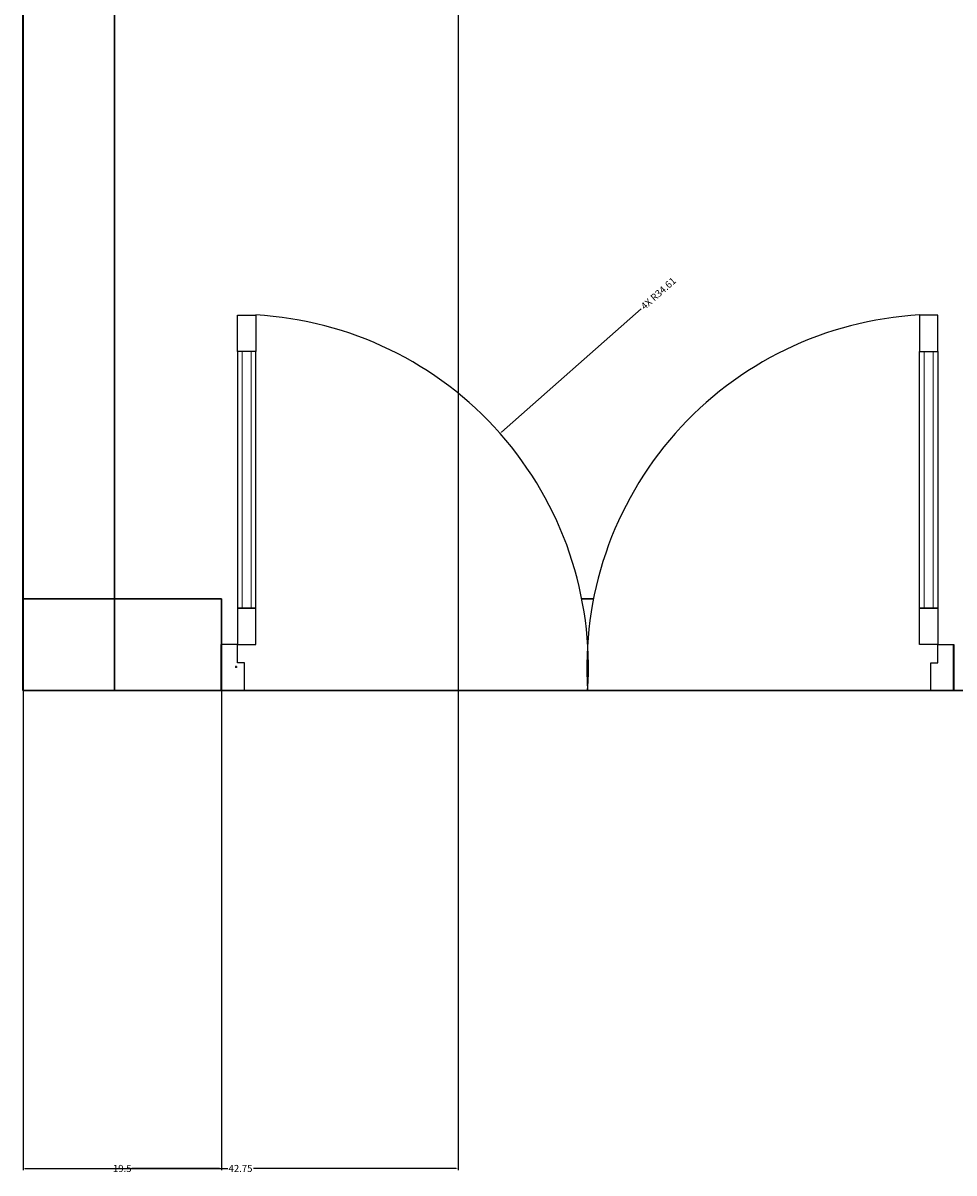
# Model space of a CAD drawing. Units: inches. Extents: x 867 to 1667, y -234 to 788.
# Tile 1 of 42: x 915 to 1006, y -234 to -121. Entities that reach past the tile are written whole.
import ezdxf

# ---------------------------------------------------------------- set-up
doc = ezdxf.new("R2010")
doc.units = ezdxf.units.IN
doc.header["$MEASUREMENT"] = 0
for name, color, linetype, lineweight in [('A-ANNO-DIMS', 2, 'Continuous', 18), ('A-Door', 150, 'Continuous', 25), ('A-Glaz', 92, 'Continuous', 18), ('A-Wall', 7, 'Continuous', 35), ('A-WALL-SITE', 8, 'Continuous', 30)]:
    doc.layers.add(name, color=color, linetype=linetype, lineweight=lineweight)
doc.layers.add('NT', color=1, linetype='Continuous')
doc.styles.get("Standard").update_dxf_attribs({"font": 'arial.ttf'})
doc.dimstyles.get("Standard").update_dxf_attribs({"dimtxt": 0.6875, "dimasz": 0.18, "dimexe": 0.18, "dimexo": 0.0625, "dimgap": 0.09, "dimtad": 0, "dimdec": 4, "dimzin": 0, "dimdsep": 46, "dimlunit": 4, "dimtxsty": 'Standard', "dimcen": 0.09, "dimadec": 0, "dimazin": 0, "dimtfac": 1, "dimtdec": 4, "dimtofl": 0, "dimtmove": 0, "dimatfit": 3, "dimfxl": 1, "dimtolj": 1, "dimtzin": 0, "dimarcsym": 0})

# ---------------------------------------------------------------- blocks, each defined once
blk = doc.blocks.new('A$C0EE93B68')
at = {"layer": 'A-Door'}
for points in [[(100, 1565), (100, 1600), (0, 1600), (0, 1550), (50, 1550), (60, 1550), (60, 1565)], [(100, 1525), (180, 1525), (180, 1565), (100, 1565)], [(180, 1525), (740, 1525), (740, 1565), (180, 1565)], [(820, 1525), (740, 1525), (740, 1565), (820, 1565)], [(100, 75), (180, 75), (180, 35), (100, 35)], [(180, 75), (740, 75), (740, 35), (180, 35)], [(820, 75), (740, 75), (740, 35), (820, 35)], [(100, 35), (100, 0), (0, 0), (0, 50), (50, 50), (60, 50), (60, 35)]]:
    blk.add_lwpolyline(points, close=True, dxfattribs=at)
at = {"layer": 'A-Glaz'}
for points in [[(180, 1535), (740, 1535), (740, 1555), (180, 1555)], [(180, 65), (740, 65), (740, 45), (180, 45)]]:
    blk.add_lwpolyline(points, close=True, dxfattribs=at)
at = {"layer": 'A-Wall'}
for p, q in [((0, 1600), (100, 1600)), ((0, 0), (100, 0))]:
    blk.add_line(p, q, dxfattribs=at)
at = {"layer": 'NT'}
for centre, start, end in [((51.6, 1567.9), 266.1547, 356.8081), ((51.6, 32.1), 3.1919, 93.8453)]:
    blk.add_arc(centre, 769.6, start, end, dxfattribs=at)
blk = doc.blocks.new('*D26')
at = {"layer": 'A-ANNO-DIMS', "color": 0, "lineweight": -2, "transparency": 16777216}
for p, q in [((914.89, -186.47), (914.89, -233.54)), ((934.39, -186.47), (934.39, -233.54)), ((915.07, -233.36), (923.68, -233.36)), ((934.21, -233.36), (925.59, -233.36))]:
    blk.add_line(p, q, dxfattribs=at)
at = {"layer": 'A-ANNO-DIMS', "color": 0, "transparency": 16777216}
for points in [[(915.07, -233.33), (915.07, -233.39), (914.89, -233.36)], [(934.21, -233.33), (934.21, -233.39), (934.39, -233.36)]]:
    blk.add_solid(points, dxfattribs=at)
at = {"layer": 'Defpoints', "color": 0, "transparency": 16777216}
for p in [(914.89, -186.41), (934.39, -186.41), (914.89, -233.36)]:
    blk.add_point(p, dxfattribs=at)
at = {"layer": 'A-ANNO-DIMS', "color": 0, "transparency": 16777216, "insert": (924.64, -233.36), "char_height": 0.688, "attachment_point": 5}
blk.add_mtext('\\A1;19.5', dxfattribs=at)
blk = doc.blocks.new('*D28')
at = {"layer": 'A-ANNO-DIMS', "color": 0, "lineweight": -2, "transparency": 16777216}
for p, q in [((914.89, 623.55), (914.89, -233.54)), ((957.64, 623.55), (957.64, -233.54)), ((915.07, -233.36), (935, -233.36)), ((957.46, -233.36), (937.53, -233.36))]:
    blk.add_line(p, q, dxfattribs=at)
at = {"layer": 'A-ANNO-DIMS', "color": 0, "transparency": 16777216}
for points in [[(915.07, -233.33), (915.07, -233.39), (914.89, -233.36)], [(957.46, -233.33), (957.46, -233.39), (957.64, -233.36)]]:
    blk.add_solid(points, dxfattribs=at)
at = {"layer": 'Defpoints', "color": 0, "transparency": 16777216}
for p in [(914.89, 623.62), (957.64, 623.62), (914.89, -233.36)]:
    blk.add_point(p, dxfattribs=at)
at = {"layer": 'A-ANNO-DIMS', "color": 0, "transparency": 16777216, "insert": (936.26, -233.36), "char_height": 0.688, "attachment_point": 5}
blk.add_mtext('\\A1;42.75', dxfattribs=at)
blk = doc.blocks.new('*D65')
at = {"layer": 'A-ANNO-DIMS', "color": 0, "lineweight": -2, "transparency": 16777216}
for p, q in [((975.63, -148.91), (961.9, -161.04)), ((935.74, -184.09), (935.92, -184.09)), ((935.83, -184.18), (935.83, -184))]:
    blk.add_line(p, q, dxfattribs=at)
at = {"layer": 'A-ANNO-DIMS', "color": 0, "transparency": 16777216}
blk.add_solid([(961.88, -161.02), (961.92, -161.06), (961.76, -161.16)], dxfattribs=at)
at = {"layer": 'Defpoints', "color": 0, "transparency": 16777216}
for p in [(961.76, -161.16), (935.83, -184.09)]:
    blk.add_point(p, dxfattribs=at)
at = {"layer": 'A-ANNO-DIMS', "color": 0, "transparency": 16777216, "insert": (977.32, -147.41), "char_height": 0.6875, "attachment_point": 5, "rotation": 41.4815}
blk.add_mtext('\\A1;4X R34.61', dxfattribs=at)

msp = doc.modelspace()

# ---------------------------------------------------------------- linework, layer by layer
at = {"layer": 'A-WALL-SITE'}
for p, q in [((914.8866, 740.617), (914.8866, -186.4081)), ((923.8866, 740.617), (923.8866, -186.4081)), ((934.3882, -177.4081), (914.8866, -177.4081)), ((934.3882, -177.4081), (934.3882, -186.4081)), ((934.3882, -177.4081), (934.3882, -186.4081)), ((970.9402, -177.4081), (969.7951, -177.4081)), ((1619.8866, -186.4081), (914.8866, -186.4081))]:
    msp.add_line(p, q, dxfattribs=at)

# ---------------------------------------------------------------- block references
at = {"layer": 'A-Door', "xscale": 0.0449743717352066, "yscale": 0.0449743717352066, "zscale": 0.0449743717352066, "rotation": 90}
msp.add_blockref('A$C0EE93B68', (1006.3472, -186.4081), dxfattribs=at)

# ---------------------------------------------------------------- dimensions: what is measured, and where the dimension line sits
at = {"layer": 'A-ANNO-DIMS'}
for p1, p2, override, picture, middle in [((957.6375, 623.617), (914.8866, 623.617), {"dimdec": 2, "dimlfac": 1, "dimrnd": 0, "dimzin": 0, "dimdsep": 46, "dimlunit": 2}, '*D28', (936.2621, -233.3581)), ((934.3882, -186.4081), (914.8866, -186.4081), {"dimdec": 1, "dimlfac": 1, "dimrnd": 0, "dimzin": 0, "dimdsep": 46, "dimlunit": 2}, '*D26', (924.6374, -233.3581))]:
    dim = msp.add_linear_dim(base=(914.8866, -233.3581), p1=p1, p2=p2, dimstyle='Standard', override=override, dxfattribs=at)
    dim.commit()
    dim.dimension.update_dxf_attribs({"geometry": picture, "text_midpoint": middle})
dim = msp.add_radius_dim(center=(935.834, -184.087), mpoint=(961.764, -161.161), text='4X <>', dimstyle='Standard', override={"dimdec": 2, "dimlfac": 1, "dimrnd": 0, "dimzin": 0, "dimdsep": 46, "dimlunit": 2}, dxfattribs=at)
dim.commit()
dim.dimension.update_dxf_attribs({"geometry": '*D65', "text_midpoint": (977.3219, -147.4055), "dimtype": 164})

doc.saveas('drawing.dxf')
